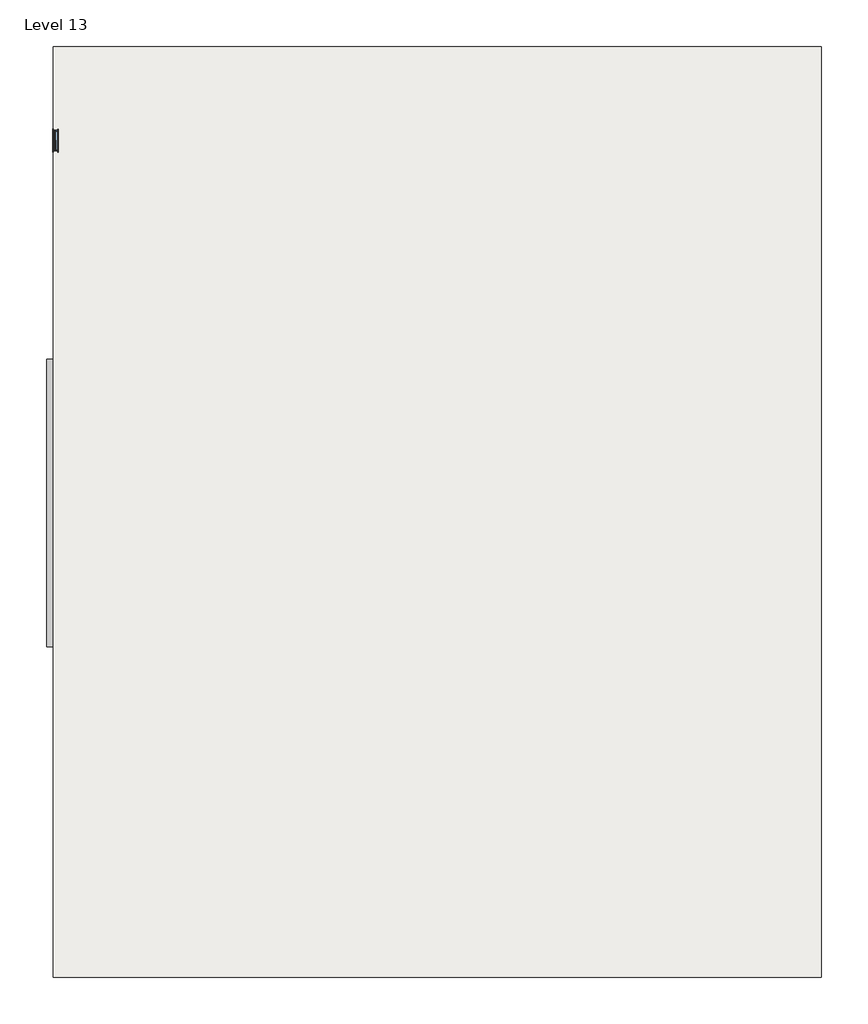
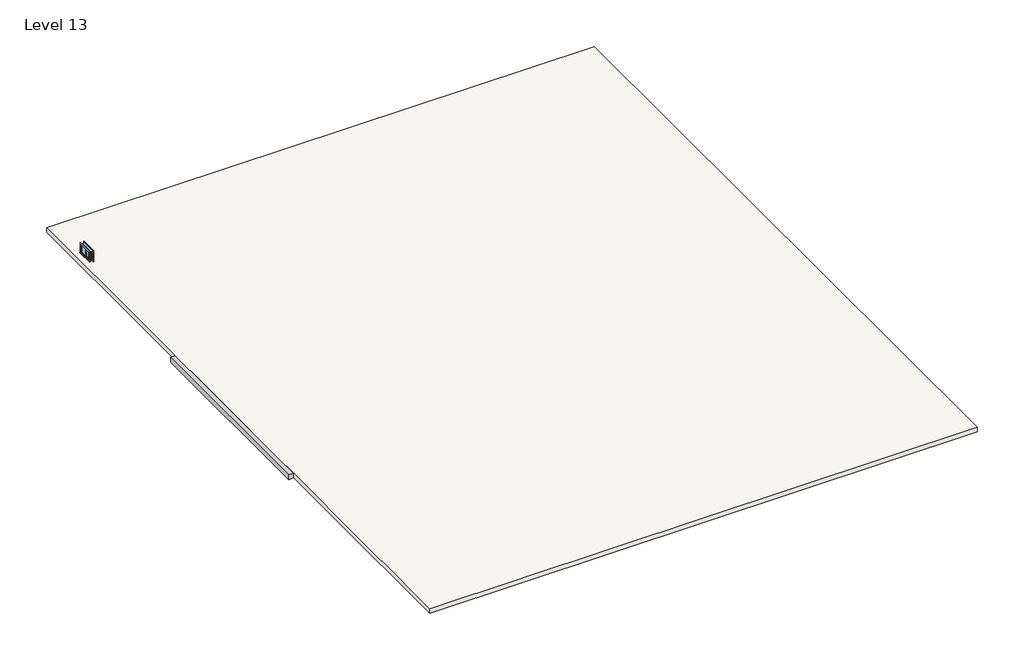
# One storey: 1 proxy, 1 slab, 1 window.
"""IFC4 building model written with IfcOpenShell, lengths in millimetres."""

from ifc_helpers import new_model, si_unit, frame, origin, place, context, project, spatial, polyline, outline, extrude, transform, mapped, element, save
from components import generic_models_17_generic_models_17_16b6177c, window_a4355bb3

model = new_model("IFC4")

# Units and contexts
model_context = context("Model", 3, world=origin())
ifc_project = project(units=[si_unit("LENGTHUNIT", "METRE", prefix="MILLI")], contexts=[model_context])

# Site, building, storey
site = spatial("IfcSite", under=ifc_project)
building = spatial("IfcBuilding", under=site)
storey = spatial("IfcBuildingStorey", under=building, Name="Level 13", Elevation=22860.0)

# Proxy
placement = place(None, origin())
generic_models_17_generic_models_17_shape = generic_models_17_generic_models_17_16b6177c(model_context)
element("IfcBuildingElementProxy", 1, Name="Generic Models 17 : Generic Models 17", ObjectType="Generic Models 17 : Generic Models 17", at=placement, inside=storey, context=model_context, shape_type="MappedRepresentation", body=[
    mapped(generic_models_17_generic_models_17_shape, transform((0.0, 0.0, 0.0), x_axis=(1.0, 0.0, 0.0), y_axis=(0.0, 1.0, 0.0), z_axis=(0.0, 0.0, 1.0))),
])

# Slab
element("IfcSlab", 2, ObjectType="Generic - 12\"", at=placement, inside=storey, context=model_context, shape_type="SweptSolid", body=[
    extrude(outline(polyline([(19165.761926, 20911.8014639), (19165.761926, -20845.7985361), (-15276.638074, -20845.7985361), (-15276.638074, 20911.8014639), (19165.761926, 20911.8014639)])), frame((0.0, 0.0, 22860.0), z_axis=(0.0, 0.0, 1.0), x_axis=(1.0, 0.0, 0.0)), (0.0, 0.0, 1.0), 304.8),
])

# Window
window_shape = window_a4355bb3(model_context)
element("IfcWindow", 3, ObjectType="Slider with Trim : 36\" x 24\"", at=placement, inside=storey, context=model_context, shape_type="MappedRepresentation", body=[
    mapped(window_shape, transform((-15175.038074, 16695.4014639, 22860.0), x_axis=(0.0, 1.0, 0.0), y_axis=(-1.0, 0.0, 0.0), z_axis=(0.0, 0.0, 1.0))),
])

save(model, "model.ifc")

# Revit data of these elements
# Type "Generic - 12\""
#   Assembly Code = "B1010"
#   Function = 0
#   Layers, outside or top first: 1' - 0" no material (function 1)
# Type "Slider with Trim : 36\" x 24\""
#   Type Mark = "23"
#   Construction Type Id = "GSP4R"
#   Assembly Code = "B2020100"
#   Analytic Construction = "1/8 in Pilkington single glazing"
#   Visual Light Transmittance = 0.9
#   Solar Heat Gain Coefficient = 0.78
#   Heat Transfer Coefficient (U) = 0.6496 BTU/(h·ft²·°F)
#   Height = 2' - 0"
#   Default Sill Height = 3' - 0"
#   Trim Projection - Ext. = 0' - 0 3/4"
#   Trim Projection - Int. = 0' - 0 3/4"
#   Trim Width - Exterior = 0' - 3 1/2"
#   Trim Width - Interior = 0' - 3 1/2"
#   Width = 3' - 0"
#   Window Inset = 0' - 0 3/4"
#   Define Thermal Properties by = 1
#   Glass Pane Material = Glass
#   Sash Material = Sash
#   Trim Exterior Material = Trim
#   Trim Interior Material = Trim
#   Wall Closure = (empty or 0)
# Element 1 (IfcBuildingElementProxy, "Generic Models 17 : Generic Models 17")
#   Phase Created = New Construction
# Element 2 (IfcSlab, "Generic - 12\"")
#   Height Offset From Level = 1' - 0"
#   Phase Created = New Construction
#   Materials on its faces: "Default Floor"
# Element 3 (IfcWindow, "Slider with Trim : 36\" x 24\"")
#   Mark = "60"
#   Phase Created = New Construction
#   Materials on its faces: "Sash", "Trim", "Glass"
# Materials
#   "Glass": class "Glass", colour RGB 0 128 192, transparency 0.75, Description = "Soda Lime Glass", Cost = 0
#   "Sash": class "Wood", colour RGB 224 178 126, transparency 0
#   "Trim": class "Wood", colour RGB 224 178 126, transparency 0
#   "Default Floor": colour RGB 128 128 128, transparency 0
